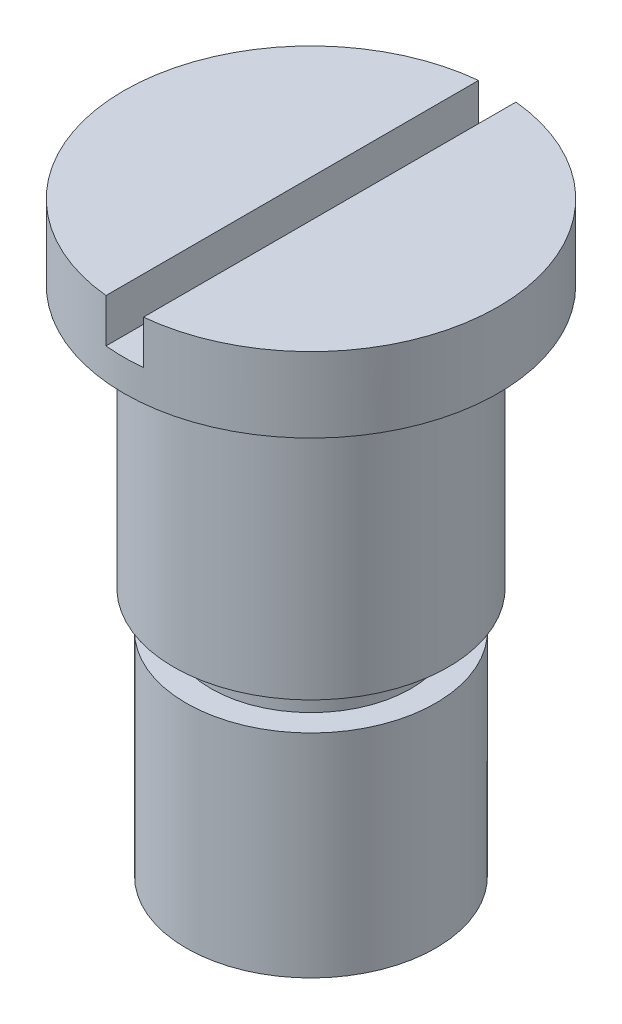
SolidWorks part; units mm, degrees
material "Plain Carbon Steel"
ref_plane "Front Plane" through (0, 0, 0) normal (0, 0, 1) x (1, 0, 0)
ref_plane "Top Plane" through (0, 0, 0) normal (0, 1, 0) x (1, 0, 0)
ref_plane "Right Plane" through (0, 0, 0) normal (1, 0, 0) x (0, 0, -1)
sketch "Lower Shank Sketch Ø20" plane through (0, 0, 0) normal (0, 1, 0) x (1, 0, 0)
  circle A0 centre (0, 0) radius 10
  dimension "D1" = 20
extrude "Lower Shank Ø20" add sketch "Lower Shank Sketch Ø20" along normal blind 17
sketch "Groove Neck Sketch Ø16" plane through (0, 17, 0) normal (0, 1, 0) x (1, 0, 0)
  circle A0 centre (0, 0) radius 8
  dimension "D1" = 16
extrude "Groove Neck Ø16" add sketch "Groove Neck Sketch Ø16" along normal blind 3
sketch "Upper Shank Sketch Ø22" plane through (0, 20, 0) normal (0, 1, 0) x (1, 0, 0)
  circle A0 centre (0, 0) radius 11
  dimension "D1" = 22
extrude "Upper Shank Ø22" add sketch "Upper Shank Sketch Ø22" along normal blind 21 contours A0
sketch "Head Sketch Ø30" plane through (0, 41, 0) normal (0, 1, 0) x (1, 0, 0)
  circle A0 centre (0, 0) radius 15
  dimension "D1" = 30
extrude "Head Ø30" add sketch "Head Sketch Ø30" along normal blind 6
sketch "Screwdriver Slot Sketch" plane through (0, 47, 0) normal (0, 1, 0) x (1, 0, 0)
  line L3 (-1.5, 16.1903) -> (1.5, 16.1903)
  line L4 (-1.5, 16.1903) -> (-1.5, -16.273)
  line L5 (-1.5, -16.273) -> (1.5, -16.273)
  line L6 (1.5, 16.1903) -> (1.5, -16.273)
  circle A0 centre (0, 0) radius 15 construction
  dimension "D1" = 3
  dimension "D2" = 1.5
  dimension "D3" = 16.1903
  dimension "D4" = 16.273
extrude "Screwdriver Slot 3x3.5" cut sketch "Screwdriver Slot Sketch" against normal blind 3.5
